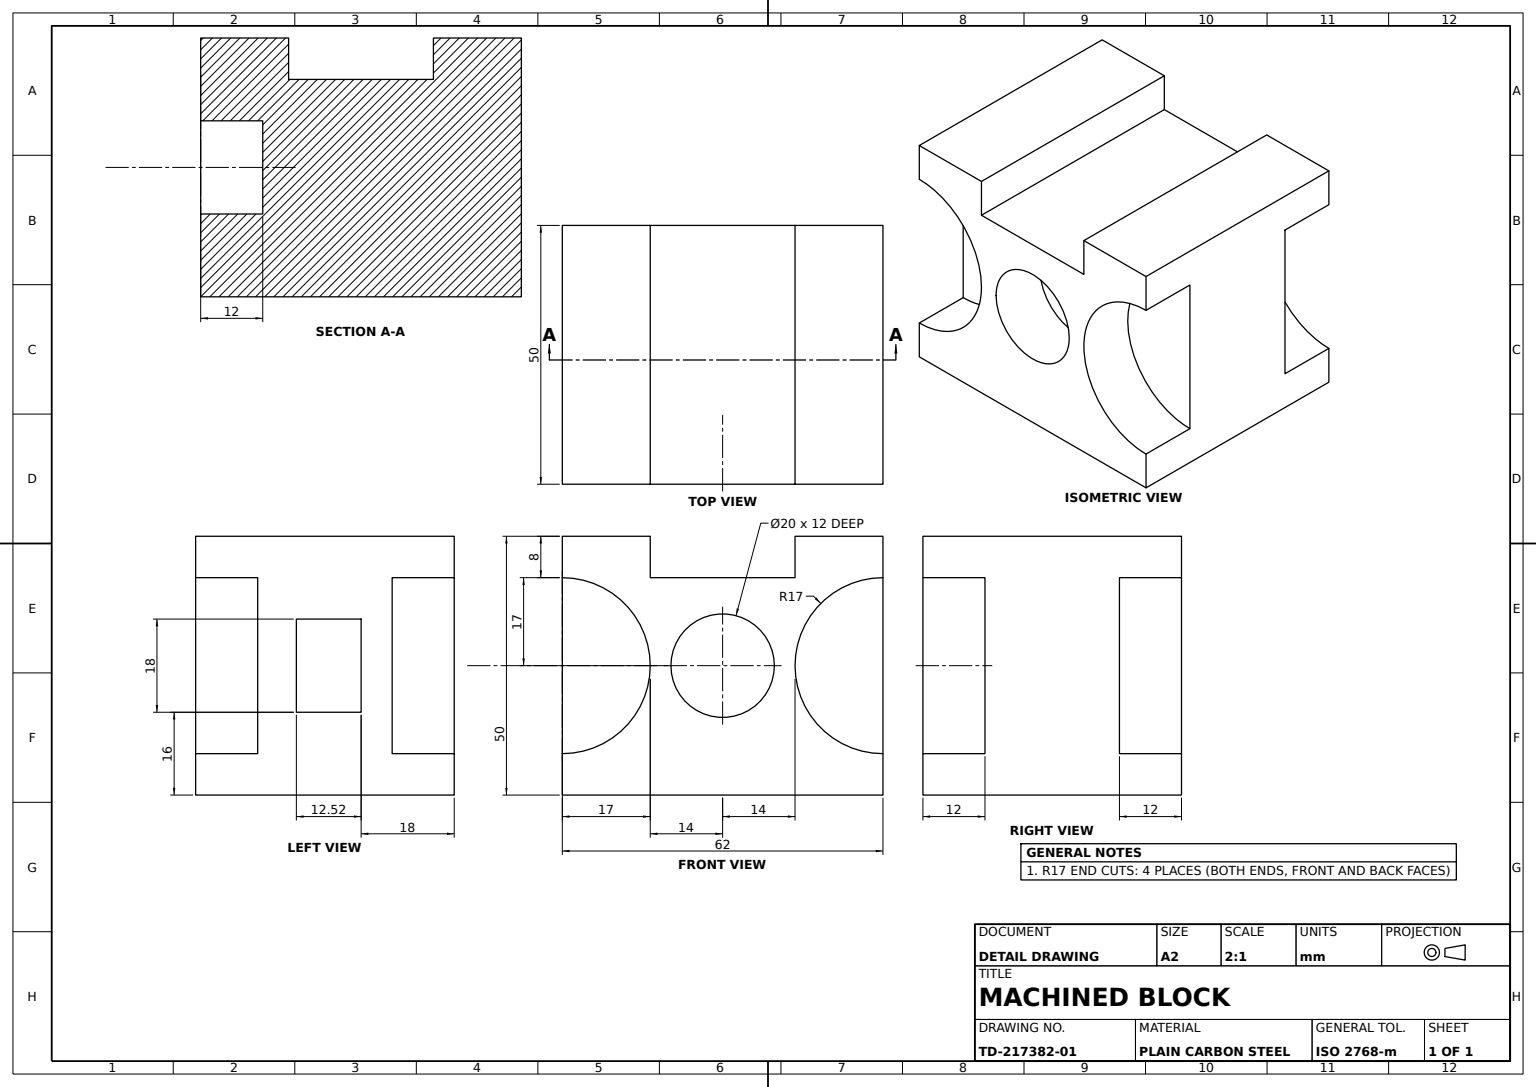
SolidWorks part; units mm, degrees
material "Plain Carbon Steel"
ref_plane "Front Plane" through (0, 0, 0) normal (0, 0, 1) x (1, 0, 0)
ref_plane "Top Plane" through (0, 0, 0) normal (0, 1, 0) x (1, 0, 0)
ref_plane "Right Plane" through (0, 0, 0) normal (1, 0, 0) x (0, 0, -1)
sketch "Block Profile 62x50" plane through (0, 0, 0) normal (0, 0, 1) x (1, 0, 0)
  line L0 (0, 0) -> (62, 0)
  line L1 (62, 0) -> (62, 50)
  line L2 (62, 50) -> (0, 50)
  line L3 (0, 50) -> (0, 0)
  dimension "D1" = 62
  dimension "D2" = 50
extrude "Base Block 62x50x50" add sketch "Block Profile 62x50" along normal blind 50
sketch "Square Cut A Profile 34x34" plane through (0, 0, 50) normal (0, 0, 1) x (1, 0, 0)
  line L0 (31, 0) -> (31, 50) construction
  line L1 (0, 0) -> (62, 0) construction
  line L2 (62, 50) -> (0, 50) construction
  line L3 (0, 25) -> (62, 25) construction
  line L4 (0, 50) -> (0, 0) construction
  line L5 (62, 0) -> (62, 50) construction
  circle A1 centre (62, 25) radius 17
  circle A2 centre (0, 25) radius 17
  dimension "D2" = 34
  dimension "D3" = 34
extrude "Square Cut A 34x34 Depth 12" cut sketch "Square Cut A Profile 34x34" against normal blind 12
sketch "Side Arc Cut A Profile" plane through (0, 0, 50) normal (0, 0, 1) x (1, 0, 0)
  line L0 (31, 50) -> (31, 0) construction
  line L1 (62, 50) -> (0, 50) construction
  line L2 (0, 0) -> (62, 0) construction
  line L3 (17, 25) -> (45, 25) construction
  line L5 (31, 42) -> (17, 42)
  line L6 (17, 42) -> (17, 50)
  line L7 (17, 50) -> (45, 50)
  line L8 (45, 50) -> (45, 42)
  line L9 (45, 42) -> (31, 42)
  arc A0 (0, 8) -> (0, 42) centre (0, 25) ccw construction
  arc A1 (62, 42) -> (62, 8) centre (62, 25) ccw construction
  dimension "D1" = 8
  dimension "D2" = 14
  dimension "D3" = 14
extrude "Side Arc Cut A" cut sketch "Side Arc Cut A Profile" against normal through all
sketch "Side Arc Cut B Profile" plane through (0, 0, 0) normal (-1, 0, 0) x (0, 0, 1)
  line L0 (25, 0) -> (25, 50) construction
  line L1 (50, 0) -> (0, 0) construction
  line L2 (50, 50) -> (0, 50) construction
  line L3 (0, 25) -> (38, 25) construction
  line L4 (0, 50) -> (0, 0) construction
  line L5 (38, 8) -> (38, 42) construction
  line L7 (25, 34) -> (19.4759, 34)
  line L8 (19.4759, 34) -> (19.4759, 16)
  line L9 (19.4759, 16) -> (32, 16)
  line L10 (32, 16) -> (32, 34)
  line L11 (32, 34) -> (25, 34)
  dimension "D1" = 7
  dimension "D2" = 5.5241
  dimension "D3" = 18
  dimension "D4" = 9
extrude "Side Arc Cut B Depth 12" cut sketch "Side Arc Cut B Profile" against normal blind 12
sketch "Square Cut B Profile 34x34" plane through (0, 0, 0) normal (0, 0, -1) x (-1, 0, 0)
  line L0 (-62, 25) -> (0, 25) construction
  line L1 (-62, 0) -> (-62, 50) construction
  line L2 (0, 50) -> (0, 0) construction
  line L3 (-31, 0) -> (-31, 42) construction
  line L4 (0, 0) -> (-62, 0) construction
  line L5 (-17, 42) -> (-45, 42) construction
  circle A0 centre (-62, 25) radius 17
  circle A1 centre (0, 25) radius 17
  dimension "D1" = 34
  dimension "D2" = 34
extrude "Square Cut B 34x34 Depth 12" cut sketch "Square Cut B Profile 34x34" against normal blind 12
sketch "Hole Profile Ø20" plane through (0, 0, 50) normal (0, 0, 1) x (1, 0, 0)
  line L0 (0, 0) -> (62, 0) construction
  line L1 (0, 42) -> (0, 8) construction
  circle A0 centre (31, 25) radius 10
  dimension "D1" = 20
  dimension "D2" = 25
  dimension "D3" = 31
extrude "Hole Ø20 Depth 12" cut sketch "Hole Profile Ø20" against normal blind 12
